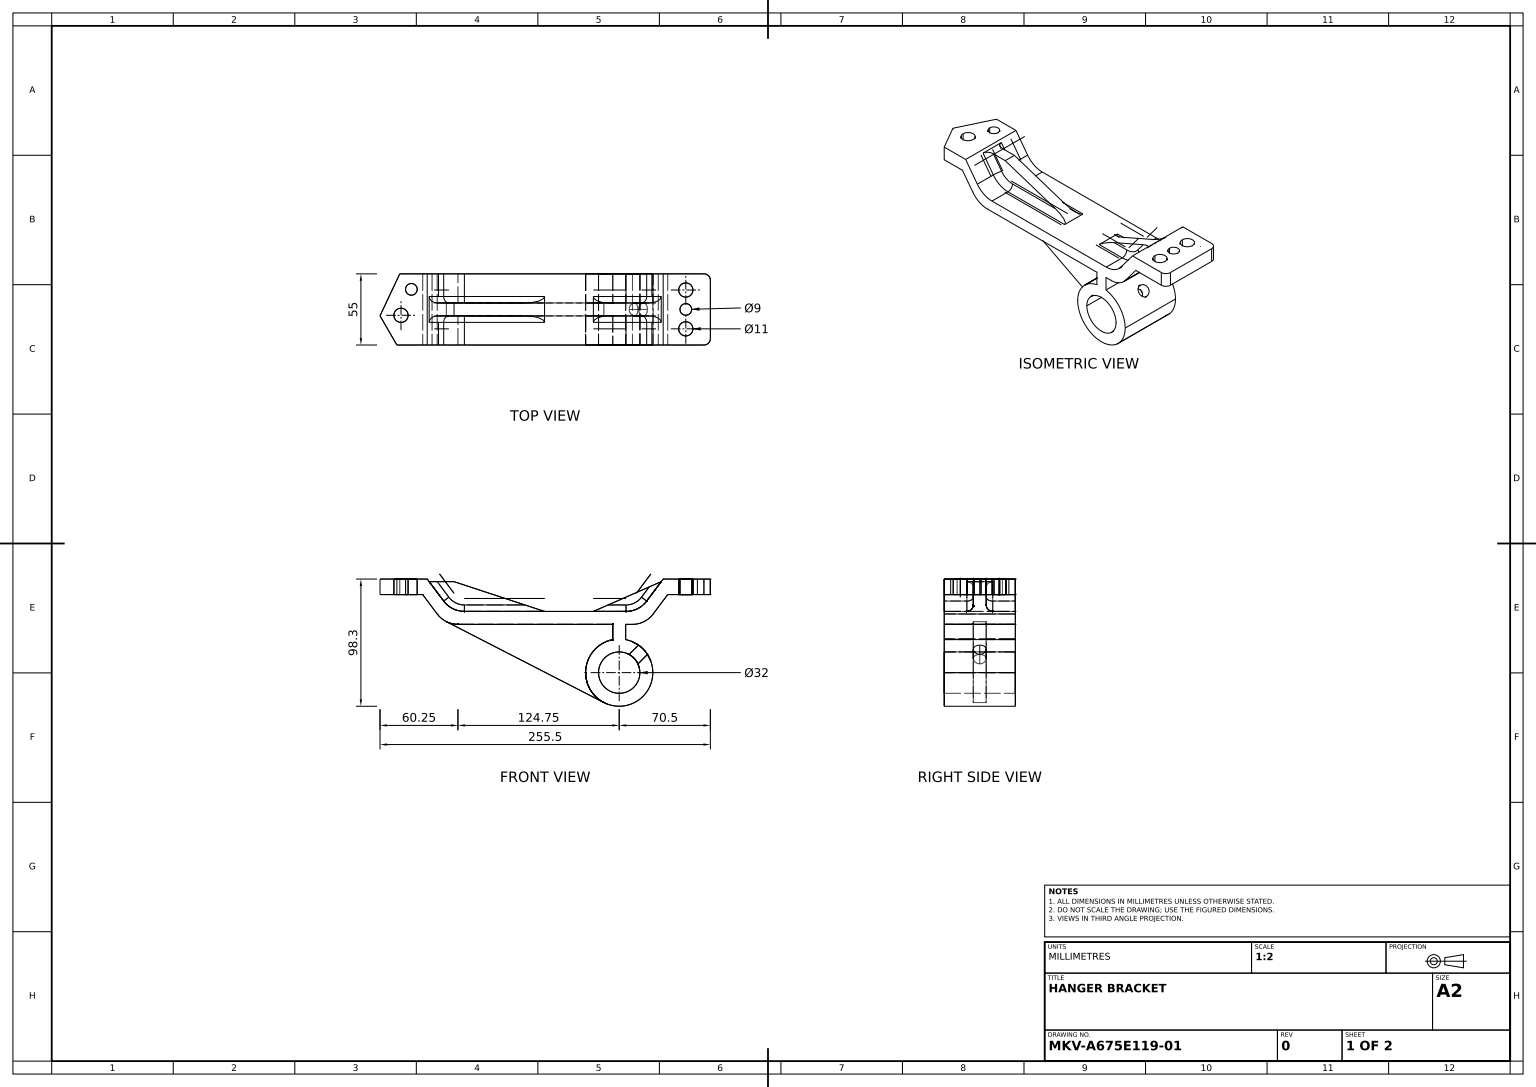
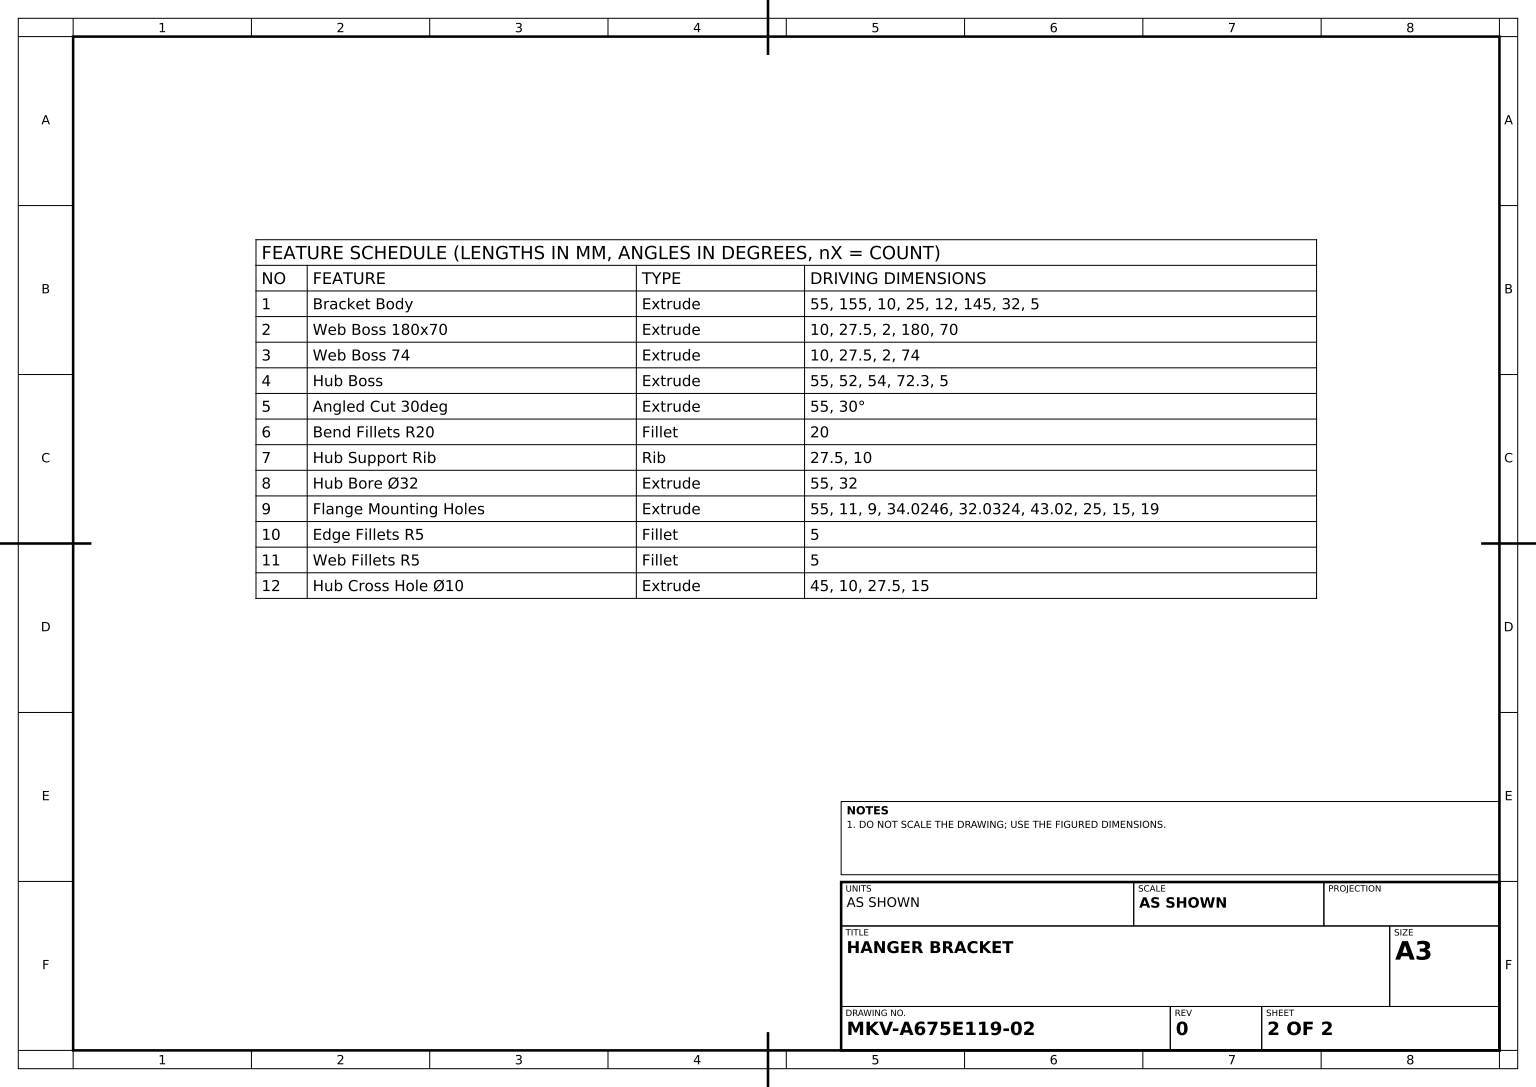
from build123d import *

# Parameters (mm, degrees)
BRACKET_BODY_DEPTH          = 55
WEB_START                   = -27.5
WEB_BOSS_180X70_DEPTH       = 5
WEB_BOSS_74_DEPTH           = 5
HUB_BOSS_SKETCH_R           = 26
HUB_BOSS_DEPTH              = 55
ANGLED_CUT_30DEG_DEPTH      = 55
BEND_FILLETS_R20_R          = 20
HUB_SUPPORT_RIB_REACH       = 218.543
SUPPORT_RIB_SKETCH_WALL_W   = 572.021051398
SUPPORT_RIB_SKETCH_WALL_H   = 10
HUB_BORE_SKETCH_R           = 16
HUB_BORE_32_DEPTH           = 55
FLANGE_HOLES_SKETCH_R       = 5.5
FLANGE_HOLES_SKETCH_R_2     = 4.5
FLANGE_MOUNTING_HOLES_DEPTH = 55
EDGE_FILLETS_R5_R           = 5
WEB_FILLETS_R5_R            = 5
CROSS_HOLE_SKETCH_R         = 5
HUB_CROSS_HOLE_10_DEPTH     = 45


with BuildPart() as part:
    # Bracket Profile Sketch → Bracket Body (new body)
    with BuildSketch(Plane.XY):
        Polygon((0, 0), (155, 0), (172.25, 23), (205.25, 23), (205.25, 35), (168.75, 35), (150, 10), (5, 10), (-13.75, 35), (-50.25, 35), (-50.25, 23), (-17.25, 23), align=None)
    extrude(amount=-BRACKET_BODY_DEPTH)

    # Web Boss 180x70 Sketch → Web Boss 180x70 (add, symmetric)
    with BuildSketch(Plane.XY.offset(WEB_START)):
        Polygon((-12.25, 33), (7, 33), (77, 10), (5, 10), align=None)
    extrude(amount=WEB_BOSS_180X70_DEPTH, both=True)

    # Web Boss 74 Sketch → Web Boss 74 (add, symmetric)
    with BuildSketch(Plane.XY.offset(WEB_START)):
        Polygon((167.25, 33), (114.75, 10), (150, 10), align=None)
    extrude(amount=WEB_BOSS_74_DEPTH, both=True)

    # Hub Boss Sketch → Hub Boss (add)
    with BuildSketch(Plane.XY):
        with Locations((134.75, -37.3)):
            Circle(HUB_BOSS_SKETCH_R)
        with BuildLine():
            ThreePointArc((129.75, -11.785298356), (134.75, -11.3), (139.75, -11.785298356))
            Line((139.75, -11.785298356), (139.75, 0))
            Line((139.75, 0), (129.75, 0))
            Line((129.75, 0), (129.75, -11.785298356))
        make_face()
    extrude(amount=-HUB_BOSS_DEPTH)

    # Angled Cut Sketch → Angled Cut 30deg (cut)
    with BuildSketch(Plane(origin=(0, 35, 0), x_dir=(1, 0, 0), z_dir=(0, 1, 0))):
        Polygon((-50.25, 55), (-50.25, 22.567969878), (-34.99199027, 55), align=None)
        Polygon((-37.220376516, 0), (-50.25, 22.567969878), (-50.25, 0), align=None)
    extrude(amount=-ANGLED_CUT_30DEG_DEPTH, mode=Mode.SUBTRACT)

    # Bend Fillets R20
    bend_fillets_r20_edges = [part.edges().sort_by_distance(p)[0] for p in [
        (5, 10, -43.75),
        (150, 10, -43.75),
        (155, 0, -27.5),
        (0, 0, -27.5),
        (5, 10, -11.25),
        (150, 10, -11.25),
    ]]
    fillet(bend_fillets_r20_edges, radius=BEND_FILLETS_R20_R)

    # Support Rib Sketch wall → Hub Support Rib (add, up to next)
    with BuildSketch(Plane(origin=(61.965504267, -29.159208524, -27.5), x_dir=(0.889610508712, -0.45671998291, 0), z_dir=(0.45671998291, 0.889610508712, 0)), mode=Mode.PRIVATE) as hub_support_rib_sk1:
        Rectangle(SUPPORT_RIB_SKETCH_WALL_W, SUPPORT_RIB_SKETCH_WALL_H)
    hub_support_rib_tool1 = extrude(hub_support_rib_sk1.sketch, amount=HUB_SUPPORT_RIB_REACH, mode=Mode.PRIVATE) - part.part
    add(hub_support_rib_tool1.solids().sort_by_distance((61.965504267, -29.159208524, -27.5))[0])

    # Hub Bore Sketch → Hub Bore Ø32 (cut)
    with BuildSketch(Plane.XY):
        with Locations((134.75, -37.3)):
            Circle(HUB_BORE_SKETCH_R)
    extrude(amount=-HUB_BORE_32_DEPTH, mode=Mode.SUBTRACT)

    # Flange Holes Sketch → Flange Mounting Holes (cut)
    with BuildSketch(Plane(origin=(0, 35, 0), x_dir=(1, 0, 0), z_dir=(0, 1, 0))):
        with Locations(Location((-34.024558742, 22.967597982, 0), (0, 0, 180))):
            Circle(FLANGE_HOLES_SKETCH_R)
        with Locations(Location((-26, 43.020043273, 0), (0, 0, 180))):
            Circle(FLANGE_HOLES_SKETCH_R_2)
        with Locations(Location((186.25, 42.5, 0), (0, 0, 180))):
            Circle(FLANGE_HOLES_SKETCH_R)
        with Locations(Location((186.25, 27.5, 0), (0, 0, 180))):
            Circle(FLANGE_HOLES_SKETCH_R_2)
        with Locations(Location((186.25, 12.5, 0), (0, 0, 180))):
            Circle(FLANGE_HOLES_SKETCH_R)
    extrude(amount=-FLANGE_MOUNTING_HOLES_DEPTH, mode=Mode.SUBTRACT)

    # Edge Fillets R5
    edge_fillets_r5_edges = [part.edges().sort_by_distance(p)[0] for p in [
        (205.25, 29, 0),
        (205.25, 29, -55),
    ]]
    fillet(edge_fillets_r5_edges, radius=EDGE_FILLETS_R5_R)

    # Web Fillets R5
    web_fillets_r5_edges = [part.edges().sort_by_distance(p)[0] for p in [
        (161.625, 25.5, -22.5),
        (161.625, 25.5, -32.5),
        (148.94427191, 12.11145618, -32.5),
        (46, 10, -32.5),
        (46, 10, -22.5),
        (148.94427191, 12.11145618, -22.5),
        (6.05572809, 12.11145618, -32.5),
        (6.05572809, 12.11145618, -22.5),
        (-6.625, 25.5, -32.5),
        (-6.625, 25.5, -22.5),
        (127.375, 10, -32.5),
        (127.375, 10, -22.5),
    ]]
    fillet(web_fillets_r5_edges, radius=WEB_FILLETS_R5_R)

    # Cross Hole Sketch → Hub Cross Hole Ø10 (cut)
    with BuildSketch(Plane(origin=(163.566905934, -8.483094066, 0), x_dir=(0.7071067811865488, -0.7071067811865462, 0), z_dir=(0.7071067811865462, 0.7071067811865488, 0))):
        with Locations(Location((0.493915353, 27.5, 0), (0, 0, 180))):
            Circle(CROSS_HOLE_SKETCH_R)
    extrude(amount=-HUB_CROSS_HOLE_10_DEPTH, mode=Mode.SUBTRACT)


solid = part.part
